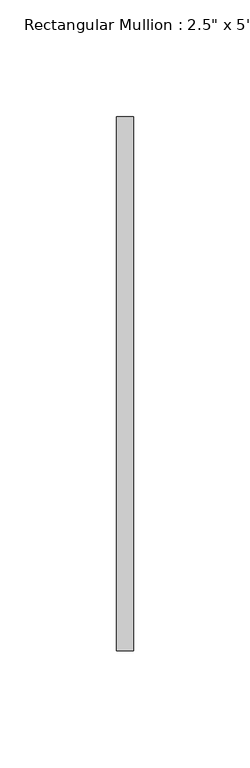
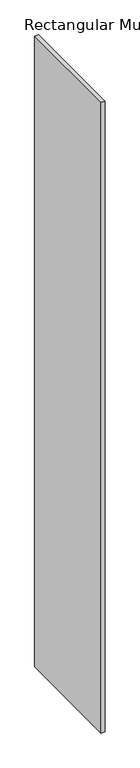
"""IFC4 building model written with IfcOpenShell, lengths in millimetres: member geometry."""

from ifc_helpers import new_model, si_unit, frame, origin, place, context, project, spatial, polyline, outline, extrude, source, transform, mapped, element, save


def member_6fc4240e(model_context):
    return source(origin(), model_context, "Body", "SweptSolid", [
        extrude(outline(polyline([(3.6195, 114.3), (3.6195, -114.3), (-3.6195, -114.3), (-3.6195, 114.3), (3.6195, 114.3)])), frame((0.0, 0.0, -1322.6415), z_axis=(0.0, 0.0, 1.0), x_axis=(1.0, 0.0, 0.0)), (0.0, 0.0, 1.0), 1322.6415),
    ])


if __name__ == "__main__":
    model = new_model("IFC4")
    model_context = context("Model", 3, world=origin())
    ifc_project = project(units=[si_unit("LENGTHUNIT", "METRE", prefix="MILLI")], contexts=[model_context])
    site = spatial("IfcSite", under=ifc_project)
    building = spatial("IfcBuilding", under=site)
    placement = place(None, origin())
    member_shape = member_6fc4240e(model_context)
    element("IfcMember", 1, ObjectType="Rectangular Mullion : 2.5\" x 5\" rectangular", at=placement, inside=building, context=model_context, shape_type="MappedRepresentation", body=[
        mapped(member_shape, transform((0.0, 0.0, 0.0), x_axis=(1.0, 0.0, 0.0), y_axis=(0.0, 1.0, 0.0), z_axis=(0.0, 0.0, 1.0))),
    ])
    save(model, "model.ifc")

# Revit data of these elements
# Type "Rectangular Mullion : 2.5\" x 5\" rectangular"
#   built-in parameter 1007304 = 0.75 (stored number, unit not read)
#   built-in parameter 1007301 = 0.011875 (stored number, unit not read)
#   built-in parameter 1007300 = 0.011875 (stored number, unit not read)
# Element 1 (IfcMember, "Rectangular Mullion : 2.5\" x 5\" rectangular")
#   Materials on its faces: "WINDOW GLASS MATERIAL"
# Materials
#   "WINDOW GLASS MATERIAL": class "Generic", colour RGB 120 120 120, transparency 0, Cost = 0
